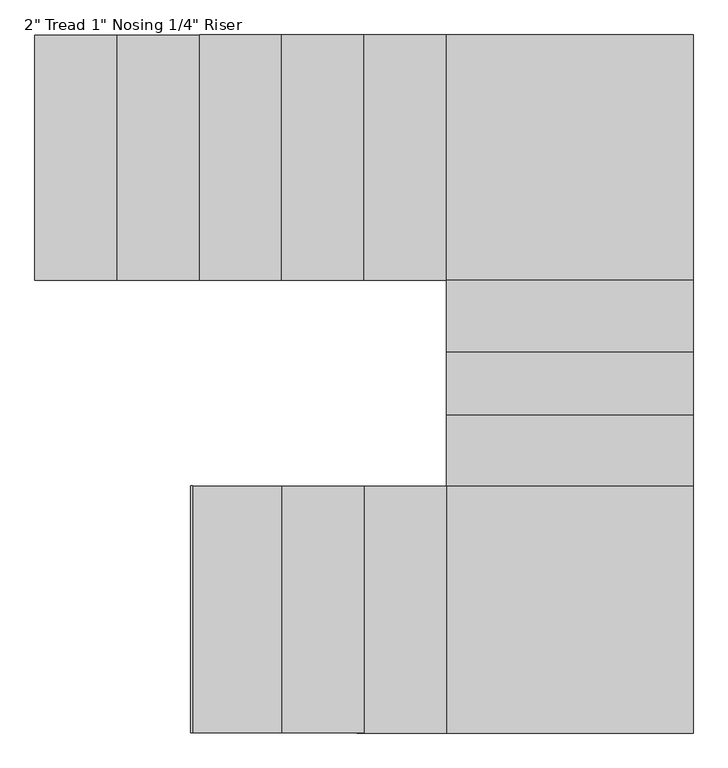
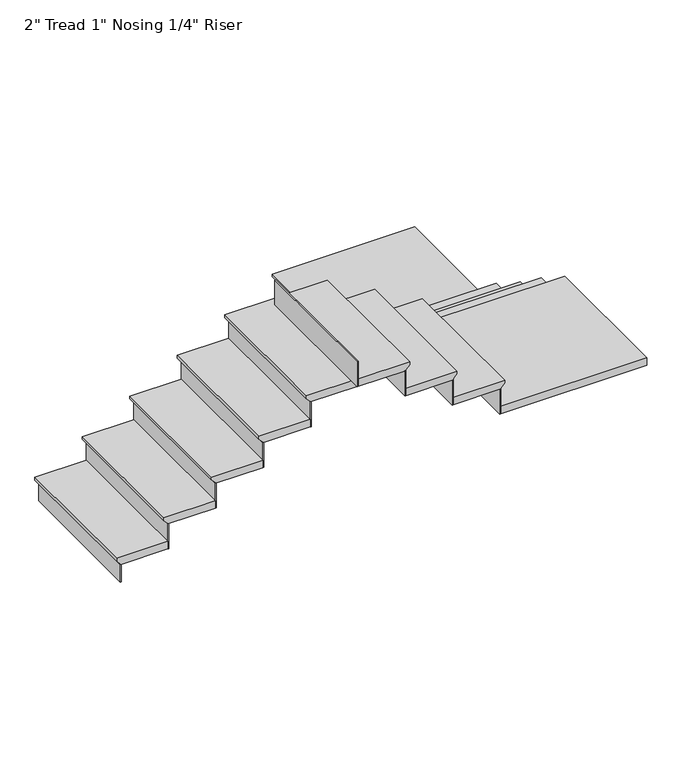
"""IFC4 building model written with IfcOpenShell, lengths in millimetres: stair flight geometry."""

from ifc_helpers import new_model, si_unit, origin, place, context, project, spatial, faceted_brep, source, transform, mapped, element, save


def stair_flight_16d52fd2(model_context):
    return source(origin(), model_context, "Body", "Brep", [
        faceted_brep([(5664.2, 3556.0, 150.2833333), (5664.2, 3556.0, 169.3333333), (5664.2, 4464.05, 169.3333333), (5664.2, 4464.05, 150.2833333), (5689.6, 3556.0, 124.8833333), (5689.6, 4464.05, 124.8833333), (5994.4, 3556.0, 169.3333333), (5994.4, 4464.05, 169.3333333), (5689.6, 4464.05, 118.5333333), (5994.4, 4464.05, 118.5333333), (5994.4, 3556.0, 118.5333333), (5689.6, 3556.0, 118.5333333)], [[[0, 1, 2, 3]], [[4, 0, 3, 5]], [[2, 1, 6, 7]], [[8, 9, 10, 11]], [[2, 7, 9, 8, 5, 3]], [[8, 11, 4, 5]], [[6, 1, 0, 4, 11, 10]], [[7, 6, 10, 9]]]),
        faceted_brep([(5689.6, 3556.0, 118.5333333), (5689.6, 3556.0, 0.0), (5695.95, 3556.0, 0.0), (5695.95, 3556.0, 118.5333333), (5689.6, 4464.05, 118.5333333), (5695.95, 4464.05, 118.5333333), (5695.95, 4464.05, 0.0), (5689.6, 4464.05, 0.0)], [[[0, 1, 2, 3]], [[4, 5, 6, 7]], [[1, 0, 4, 7]], [[2, 1, 7, 6]], [[3, 2, 6, 5]], [[0, 3, 5, 4]]]),
        faceted_brep([(5994.4, 3556.0, 287.8666667), (5994.4, 3556.0, 118.5333333), (6000.75, 3556.0, 118.5333333), (6000.75, 3556.0, 287.8666667), (5994.4, 4464.05, 287.8666667), (6000.75, 4464.05, 287.8666667), (6000.75, 4464.05, 118.5333333), (5994.4, 4464.05, 118.5333333)], [[[0, 1, 2, 3]], [[4, 5, 6, 7]], [[1, 0, 4, 7]], [[2, 1, 7, 6]], [[3, 2, 6, 5]], [[0, 3, 5, 4]]]),
        faceted_brep([(5969.0, 4464.05, 338.6666667), (5969.0, 3556.0, 338.6666667), (6299.2, 3556.0, 338.6666667), (6299.2, 4464.05, 338.6666667), (5994.4, 4464.05, 287.8666667), (6299.2, 4464.05, 287.8666667), (6299.2, 3556.0, 287.8666667), (5994.4, 3556.0, 287.8666667), (5994.4, 4464.05, 294.2166667), (5969.0, 4464.05, 319.6166667), (5994.4, 3556.0, 294.2166667), (5969.0, 3556.0, 319.6166667)], [[[0, 1, 2, 3]], [[4, 5, 6, 7]], [[0, 3, 5, 4, 8, 9]], [[4, 7, 10, 8]], [[2, 1, 11, 10, 7, 6]], [[3, 2, 6, 5]], [[11, 1, 0, 9]], [[10, 11, 9, 8]]]),
        faceted_brep([(6299.2, 3556.0, 457.2), (6299.2, 3556.0, 287.8666667), (6305.55, 3556.0, 287.8666667), (6305.55, 3556.0, 457.2), (6299.2, 4464.05, 457.2), (6305.55, 4464.05, 457.2), (6305.55, 4464.05, 287.8666667), (6299.2, 4464.05, 287.8666667)], [[[0, 1, 2, 3]], [[4, 5, 6, 7]], [[1, 0, 4, 7]], [[2, 1, 7, 6]], [[3, 2, 6, 5]], [[0, 3, 5, 4]]]),
        faceted_brep([(6273.8, 4464.05, 508.0), (6273.8, 3556.0, 508.0), (6604.0, 3556.0, 508.0), (6604.0, 4464.05, 508.0), (6299.2, 4464.05, 457.2), (6604.0, 4464.05, 457.2), (6604.0, 3556.0, 457.2), (6299.2, 3556.0, 457.2), (6299.2, 4464.05, 463.55), (6273.8, 4464.05, 488.95), (6299.2, 3556.0, 463.55), (6273.8, 3556.0, 488.95)], [[[0, 1, 2, 3]], [[4, 5, 6, 7]], [[0, 3, 5, 4, 8, 9]], [[4, 7, 10, 8]], [[2, 1, 11, 10, 7, 6]], [[3, 2, 6, 5]], [[11, 1, 0, 9]], [[10, 11, 9, 8]]]),
        faceted_brep([(6604.0, 3556.0, 626.5333333), (6604.0, 3556.0, 457.2), (6610.35, 3556.0, 457.2), (6610.35, 3556.0, 626.5333333), (6604.0, 4464.05, 626.5333333), (6610.35, 4464.05, 626.5333333), (6610.35, 4464.05, 457.2), (6604.0, 4464.05, 457.2)], [[[0, 1, 2, 3]], [[4, 5, 6, 7]], [[1, 0, 4, 7]], [[2, 1, 7, 6]], [[3, 2, 6, 5]], [[0, 3, 5, 4]]]),
        faceted_brep([(6578.6, 4464.05, 677.3333333), (6578.6, 3556.0, 677.3333333), (6908.8, 3556.0, 677.3333333), (6908.8, 4464.05, 677.3333333), (6604.0, 4464.05, 626.5333333), (6908.8, 4464.05, 626.5333333), (6908.8, 3556.0, 626.5333333), (6604.0, 3556.0, 626.5333333), (6604.0, 4464.05, 632.8833333), (6578.6, 4464.05, 658.2833333), (6604.0, 3556.0, 632.8833333), (6578.6, 3556.0, 658.2833333)], [[[0, 1, 2, 3]], [[4, 5, 6, 7]], [[0, 3, 5, 4, 8, 9]], [[4, 7, 10, 8]], [[2, 1, 11, 10, 7, 6]], [[3, 2, 6, 5]], [[11, 1, 0, 9]], [[10, 11, 9, 8]]]),
        faceted_brep([(6908.8, 3556.0, 795.8666667), (6908.8, 3556.0, 626.5333333), (6915.15, 3556.0, 626.5333333), (6915.15, 3556.0, 795.8666667), (6908.8, 4464.05, 795.8666667), (6915.15, 4464.05, 795.8666667), (6915.15, 4464.05, 626.5333333), (6908.8, 4464.05, 626.5333333)], [[[0, 1, 2, 3]], [[4, 5, 6, 7]], [[1, 0, 4, 7]], [[2, 1, 7, 6]], [[3, 2, 6, 5]], [[0, 3, 5, 4]]]),
        faceted_brep([(6883.4, 4464.05, 846.6666667), (6883.4, 3556.0, 846.6666667), (7213.6, 3556.0, 846.6666667), (7213.6, 4464.05, 846.6666667), (6908.8, 4464.05, 795.8666667), (7213.6, 4464.05, 795.8666667), (7213.6, 3556.0, 795.8666667), (6908.8, 3556.0, 795.8666667), (6908.8, 4464.05, 802.2166667), (6883.4, 4464.05, 827.6166667), (6908.8, 3556.0, 802.2166667), (6883.4, 3556.0, 827.6166667)], [[[0, 1, 2, 3]], [[4, 5, 6, 7]], [[0, 3, 5, 4, 8, 9]], [[4, 7, 10, 8]], [[2, 1, 11, 10, 7, 6]], [[3, 2, 6, 5]], [[11, 1, 0, 9]], [[10, 11, 9, 8]]]),
        faceted_brep([(7213.6, 3556.0, 965.2), (7213.6, 3556.0, 795.8666667), (7219.95, 3556.0, 795.8666667), (7219.95, 3556.0, 965.2), (7213.6, 4464.05, 965.2), (7219.95, 4464.05, 965.2), (7219.95, 4464.05, 795.8666667), (7213.6, 4464.05, 795.8666667)], [[[0, 1, 2, 3]], [[4, 5, 6, 7]], [[1, 0, 4, 7]], [[2, 1, 7, 6]], [[3, 2, 6, 5]], [[0, 3, 5, 4]]]),
        faceted_brep([(8102.6, 3530.6, 1016.0), (8102.6, 4464.05, 1016.0), (7188.2, 4464.05, 1016.0), (7188.2, 3530.6, 1016.0), (8102.6, 4464.05, 965.2), (8102.6, 3530.6, 965.2), (7188.2, 3530.6, 965.2), (7188.2, 3556.0, 965.2), (7213.6, 3556.0, 965.2), (7213.6, 4464.05, 965.2), (7213.6, 4464.05, 971.55), (7188.2, 4464.05, 996.95), (7213.6, 3556.0, 971.55), (7188.2, 3556.0, 996.95)], [[[0, 1, 2, 3]], [[4, 5, 6, 7, 8, 9]], [[1, 0, 5, 4]], [[2, 1, 4, 9, 10, 11]], [[9, 8, 12, 10]], [[8, 7, 13, 12]], [[3, 2, 11, 13, 7, 6]], [[0, 3, 6, 5]], [[11, 10, 12, 13]]]),
        faceted_brep([(7188.2, 3530.6, 1134.5333333), (7188.2, 3530.6, 965.2), (7188.2, 3524.25, 965.2), (7188.2, 3524.25, 1134.5333333), (8102.6, 3530.6, 1134.5333333), (8102.6, 3524.25, 1134.5333333), (8102.6, 3524.25, 965.2), (8102.6, 3530.6, 965.2)], [[[0, 1, 2, 3]], [[4, 5, 6, 7]], [[1, 0, 4, 7]], [[2, 1, 7, 6]], [[3, 2, 6, 5]], [[0, 3, 5, 4]]]),
        faceted_brep([(8102.6, 3556.0, 1185.3333333), (7188.2, 3556.0, 1185.3333333), (7188.2, 3264.1808604, 1185.3333333), (8102.6, 3264.1808604, 1185.3333333), (8102.6, 3530.6, 1134.5333333), (8102.6, 3264.1808604, 1134.5333333), (7188.2, 3264.1808604, 1134.5333333), (7188.2, 3530.6, 1134.5333333), (8102.6, 3530.6, 1140.8833333), (8102.6, 3556.0, 1166.2833333), (7188.2, 3530.6, 1140.8833333), (7188.2, 3556.0, 1166.2833333)], [[[0, 1, 2, 3]], [[4, 5, 6, 7]], [[0, 3, 5, 4, 8, 9]], [[4, 7, 10, 8]], [[2, 1, 11, 10, 7, 6]], [[3, 2, 6, 5]], [[11, 1, 0, 9]], [[10, 11, 9, 8]]]),
        faceted_brep([(7188.2, 3264.1808604, 1303.8666667), (7188.2, 3264.1808604, 1134.5333333), (7188.2, 3257.8308604, 1134.5333333), (7188.2, 3257.8308604, 1303.8666667), (8102.6, 3264.1808604, 1303.8666667), (8102.6, 3257.8308604, 1303.8666667), (8102.6, 3257.8308604, 1134.5333333), (8102.6, 3264.1808604, 1134.5333333)], [[[0, 1, 2, 3]], [[4, 5, 6, 7]], [[1, 0, 4, 7]], [[2, 1, 7, 6]], [[3, 2, 6, 5]], [[0, 3, 5, 4]]]),
        faceted_brep([(8102.6, 3289.5808604, 1354.6666667), (7188.2, 3289.5808604, 1354.6666667), (7188.2, 3031.2766234, 1354.6666667), (8102.6, 3031.2766234, 1354.6666667), (8102.6, 3264.1808604, 1303.8666667), (8102.6, 3031.2766234, 1303.8666667), (7188.2, 3031.2766234, 1303.8666667), (7188.2, 3264.1808604, 1303.8666667), (8102.6, 3264.1808604, 1310.2166667), (8102.6, 3289.5808604, 1335.6166667), (7188.2, 3264.1808604, 1310.2166667), (7188.2, 3289.5808604, 1335.6166667)], [[[0, 1, 2, 3]], [[4, 5, 6, 7]], [[0, 3, 5, 4, 8, 9]], [[4, 7, 10, 8]], [[2, 1, 11, 10, 7, 6]], [[3, 2, 6, 5]], [[11, 1, 0, 9]], [[10, 11, 9, 8]]]),
        faceted_brep([(7188.2, 3031.2766234, 1473.2), (7188.2, 3031.2766234, 1303.8666667), (7188.2, 3024.9266234, 1303.8666667), (7188.2, 3024.9266234, 1473.2), (8102.6, 3031.2766234, 1473.2), (8102.6, 3024.9266234, 1473.2), (8102.6, 3024.9266234, 1303.8666667), (8102.6, 3031.2766234, 1303.8666667)], [[[0, 1, 2, 3]], [[4, 5, 6, 7]], [[1, 0, 4, 7]], [[2, 1, 7, 6]], [[3, 2, 6, 5]], [[0, 3, 5, 4]]]),
        faceted_brep([(8102.6, 3056.6766234, 1524.0), (7188.2, 3056.6766234, 1524.0), (7188.2, 2768.6, 1524.0), (8102.6, 2768.6, 1524.0), (8102.6, 3031.2766234, 1473.2), (8102.6, 2768.6, 1473.2), (7188.2, 2768.6, 1473.2), (7188.2, 3031.2766234, 1473.2), (8102.6, 3031.2766234, 1479.55), (8102.6, 3056.6766234, 1504.95), (7188.2, 3031.2766234, 1479.55), (7188.2, 3056.6766234, 1504.95)], [[[0, 1, 2, 3]], [[4, 5, 6, 7]], [[0, 3, 5, 4, 8, 9]], [[4, 7, 10, 8]], [[2, 1, 11, 10, 7, 6]], [[3, 2, 6, 5]], [[11, 1, 0, 9]], [[10, 11, 9, 8]]]),
        faceted_brep([(7188.2, 2768.6, 1642.5333333), (7188.2, 2768.6, 1473.2), (7188.2, 2762.25, 1473.2), (7188.2, 2762.25, 1642.5333333), (8102.6, 2768.6, 1642.5333333), (8102.6, 2762.25, 1642.5333333), (8102.6, 2762.25, 1473.2), (8102.6, 2768.6, 1473.2)], [[[0, 1, 2, 3]], [[4, 5, 6, 7]], [[1, 0, 4, 7]], [[2, 1, 7, 6]], [[3, 2, 6, 5]], [[0, 3, 5, 4]]]),
        faceted_brep([(7162.8, 1879.6, 1693.3333333), (8102.6, 1879.6, 1693.3333333), (8102.6, 2794.0, 1693.3333333), (7162.8, 2794.0, 1693.3333333), (8102.6, 1879.6, 1642.5333333), (7162.8, 1879.6, 1642.5333333), (7162.8, 2794.0, 1642.5333333), (7188.2, 2794.0, 1642.5333333), (7188.2, 2768.6, 1642.5333333), (8102.6, 2768.6, 1642.5333333), (8102.6, 2768.6, 1648.8833333), (8102.6, 2794.0, 1674.2833333), (7188.2, 2768.6, 1648.8833333), (7188.2, 2794.0, 1674.2833333)], [[[0, 1, 2, 3]], [[4, 5, 6, 7, 8, 9]], [[1, 0, 5, 4]], [[2, 1, 4, 9, 10, 11]], [[9, 8, 12, 10]], [[8, 7, 13, 12]], [[3, 2, 11, 13, 7, 6]], [[0, 3, 6, 5]], [[11, 10, 12, 13]]]),
        faceted_brep([(7162.8, 2794.0, 1811.8666667), (7162.8, 2794.0, 1642.5333333), (7156.45, 2794.0, 1642.5333333), (7156.45, 2794.0, 1811.8666667), (7162.8, 1879.6, 1811.8666667), (7156.45, 1879.6, 1811.8666667), (7156.45, 1879.6, 1642.5333333), (7162.8, 1879.6, 1642.5333333)], [[[0, 1, 2, 3]], [[4, 5, 6, 7]], [[1, 0, 4, 7]], [[2, 1, 7, 6]], [[3, 2, 6, 5]], [[0, 3, 5, 4]]]),
        faceted_brep([(7188.2, 1879.6, 1862.6666667), (7188.2, 2794.0, 1862.6666667), (6857.3405542, 2794.0, 1862.6666667), (6857.3405542, 1879.6, 1862.6666667), (7162.8, 1879.6, 1811.8666667), (6857.3405542, 1879.6, 1811.8666667), (6857.3405542, 2794.0, 1811.8666667), (7162.8, 2794.0, 1811.8666667), (7162.8, 1879.6, 1818.2166667), (7188.2, 1879.6, 1843.6166667), (7162.8, 2794.0, 1818.2166667), (7188.2, 2794.0, 1843.6166667)], [[[0, 1, 2, 3]], [[4, 5, 6, 7]], [[0, 3, 5, 4, 8, 9]], [[4, 7, 10, 8]], [[2, 1, 11, 10, 7, 6]], [[3, 2, 6, 5]], [[11, 1, 0, 9]], [[10, 11, 9, 8]]]),
        faceted_brep([(6857.3405542, 2794.0, 1981.2), (6857.3405542, 2794.0, 1811.8666667), (6850.9905542, 2794.0, 1811.8666667), (6850.9905542, 2794.0, 1981.2), (6857.3405542, 1879.6, 1981.2), (6850.9905542, 1879.6, 1981.2), (6850.9905542, 1879.6, 1811.8666667), (6857.3405542, 1879.6, 1811.8666667)], [[[0, 1, 2, 3]], [[4, 5, 6, 7]], [[1, 0, 4, 7]], [[2, 1, 7, 6]], [[3, 2, 6, 5]], [[0, 3, 5, 4]]]),
        faceted_brep([(6882.7405542, 1879.6, 2032.0), (6882.7405542, 2794.0, 2032.0), (6552.5405542, 2794.0, 2032.0), (6552.5405542, 1879.6, 2032.0), (6857.3405542, 1879.6, 1981.2), (6552.5405542, 1879.6, 1981.2), (6552.5405542, 2794.0, 1981.2), (6857.3405542, 2794.0, 1981.2), (6857.3405542, 1879.6, 1987.55), (6882.7405542, 1879.6, 2012.95), (6857.3405542, 2794.0, 1987.55), (6882.7405542, 2794.0, 2012.95)], [[[0, 1, 2, 3]], [[4, 5, 6, 7]], [[0, 3, 5, 4, 8, 9]], [[4, 7, 10, 8]], [[2, 1, 11, 10, 7, 6]], [[3, 2, 6, 5]], [[11, 1, 0, 9]], [[10, 11, 9, 8]]]),
        faceted_brep([(6552.5405542, 2794.0, 2150.5333333), (6552.5405542, 2794.0, 1981.2), (6546.1905542, 2794.0, 1981.2), (6546.1905542, 2794.0, 2150.5333333), (6552.5405542, 1879.6, 2150.5333333), (6546.1905542, 1879.6, 2150.5333333), (6546.1905542, 1879.6, 1981.2), (6552.5405542, 1879.6, 1981.2)], [[[0, 1, 2, 3]], [[4, 5, 6, 7]], [[1, 0, 4, 7]], [[2, 1, 7, 6]], [[3, 2, 6, 5]], [[0, 3, 5, 4]]]),
        faceted_brep([(6247.7405542, 2794.0, 2319.8666667), (6247.7405542, 2794.0, 2150.5333333), (6241.3905542, 2794.0, 2150.5333333), (6241.3905542, 2794.0, 2319.8666667), (6247.7405542, 1879.6, 2319.8666667), (6241.3905542, 1879.6, 2319.8666667), (6241.3905542, 1879.6, 2150.5333333), (6247.7405542, 1879.6, 2150.5333333)], [[[0, 1, 2, 3]], [[4, 5, 6, 7]], [[1, 0, 4, 7]], [[2, 1, 7, 6]], [[3, 2, 6, 5]], [[0, 3, 5, 4]]]),
        faceted_brep([(6577.9405542, 1879.6, 2201.3333333), (6577.9405542, 2794.0, 2201.3333333), (6247.7405542, 2794.0, 2201.3333333), (6247.7405542, 1879.6, 2201.3333333), (6552.5405542, 1879.6, 2150.5333333), (6247.7405542, 1879.6, 2150.5333333), (6247.7405542, 2794.0, 2150.5333333), (6552.5405542, 2794.0, 2150.5333333), (6552.5405542, 1879.6, 2156.8833333), (6577.9405542, 1879.6, 2182.2833333), (6552.5405542, 2794.0, 2156.8833333), (6577.9405542, 2794.0, 2182.2833333)], [[[0, 1, 2, 3]], [[4, 5, 6, 7]], [[0, 3, 5, 4, 8, 9]], [[4, 7, 10, 8]], [[2, 1, 11, 10, 7, 6]], [[3, 2, 6, 5]], [[11, 1, 0, 9]], [[10, 11, 9, 8]]]),
    ])


if __name__ == "__main__":
    model = new_model("IFC4")
    model_context = context("Model", 3, world=origin())
    ifc_project = project(units=[si_unit("LENGTHUNIT", "METRE", prefix="MILLI")], contexts=[model_context])
    site = spatial("IfcSite", under=ifc_project)
    building = spatial("IfcBuilding", under=site)
    placement = place(None, origin())
    stair_flight_shape = stair_flight_16d52fd2(model_context)
    element("IfcStairFlight", 1, ObjectType="2\" Tread 1\" Nosing 1/4\" Riser", at=placement, inside=building, context=model_context, shape_type="MappedRepresentation", body=[
        mapped(stair_flight_shape, transform((0.0, 0.0, 0.0), x_axis=(1.0, 0.0, 0.0), y_axis=(0.0, 1.0, 0.0), z_axis=(0.0, 0.0, 1.0))),
    ])
    save(model, "model.ifc")
